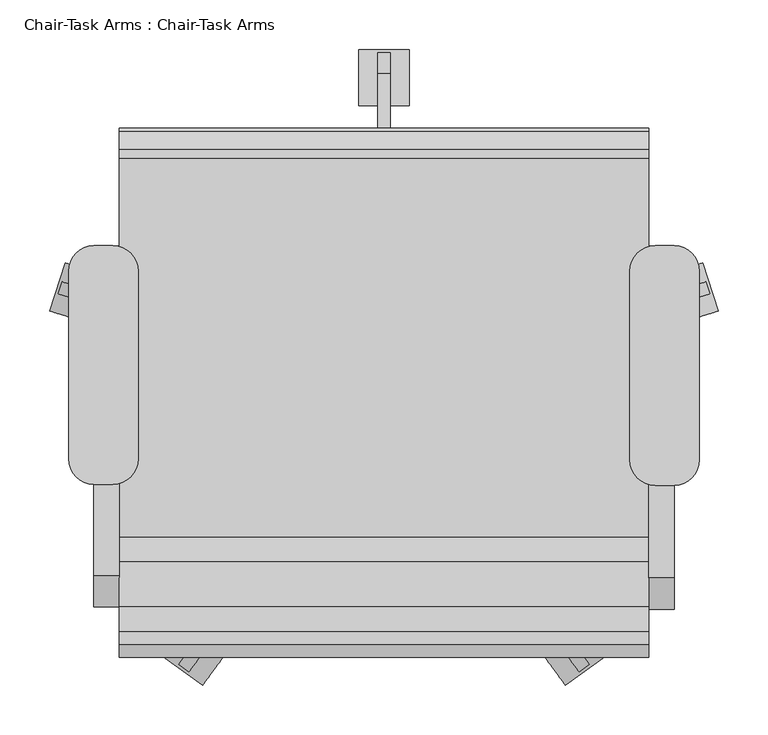
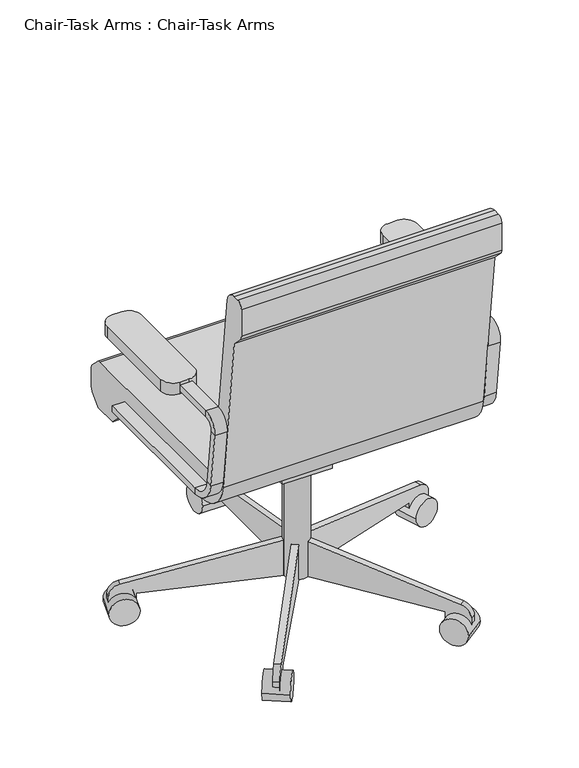
"""IFC4 building model written with IfcOpenShell, lengths in millimetres: furniture geometry, Chair-Task Arms : Chair-Task Arms."""

from ifc_helpers import new_model, si_unit, point, frame, frame_2d, origin, place, context, project, spatial, polyline, circle_curve, trimmed, segment, composite_curve, outline, extrude, source, transform, mapped, element, save
from ifc_brep_helpers import plane_surface, cylinder_surface, revolved_surface, advanced_brep


def chair_task_arms_chair_task_arms_fa5a08ef(model_context):
    return source(origin(), model_context, "Body", "SolidModel", [
        extrude(outline(composite_curve([segment(polyline([(433.0908197, -74.2028048), (414.0408197, -74.2028048)]), True, "CONTINUOUS"), segment(trimmed(circle_curve(frame_2d((414.0408197, -48.8028048)), 25.4), [point((414.0408197, -74.2028048))], [point((388.6408197, -48.8028048))], False, "CARTESIAN"), True, "CONTINUOUS"), segment(polyline([(388.6408197, -48.8028048), (388.6408197, 141.6319091)]), True, "CONTINUOUS"), segment(trimmed(circle_curve(frame_2d((414.0408197, 141.6319091)), 25.4), [point((388.6408197, 141.6319091))], [point((414.0408197, 167.0319091))], False, "CARTESIAN"), True, "CONTINUOUS"), segment(polyline([(414.0408197, 167.0319091), (433.0908197, 167.0319091)]), True, "CONTINUOUS"), segment(trimmed(circle_curve(frame_2d((433.0908197, 141.6319091)), 25.4), [point((433.0908197, 167.0319091))], [point((458.4908197, 141.6319091))], False, "CARTESIAN"), True, "CONTINUOUS"), segment(polyline([(458.4908197, 141.6319091), (458.4908197, -48.8028048)]), True, "CONTINUOUS"), segment(trimmed(circle_curve(frame_2d((433.0908197, -48.8028048)), 25.4), [point((458.4908197, -48.8028048))], [point((433.0908197, -74.2028048))], False, "CARTESIAN"), True, "CONTINUOUS")], self_intersect=False)), frame((0.0, 0.0, 596.9), z_axis=(0.0, 0.0, 1.0), x_axis=(1.0, 0.0, 0.0)), (0.0, 0.0, 1.0), 25.4),
        extrude(outline(composite_curve([segment(polyline([(-132.0591803, -73.1575984), (-151.1091803, -73.1575984)]), True, "CONTINUOUS"), segment(trimmed(circle_curve(frame_2d((-151.1091803, -47.7575984)), 25.4), [point((-151.1091803, -73.1575984))], [point((-176.5091803, -47.7575984))], False, "CARTESIAN"), True, "CONTINUOUS"), segment(polyline([(-176.5091803, -47.7575984), (-176.5091803, 141.6319091)]), True, "CONTINUOUS"), segment(trimmed(circle_curve(frame_2d((-151.1091803, 141.6319091)), 25.4), [point((-176.5091803, 141.6319091))], [point((-151.1091803, 167.0319091))], False, "CARTESIAN"), True, "CONTINUOUS"), segment(polyline([(-151.1091803, 167.0319091), (-132.0591803, 167.0319091)]), True, "CONTINUOUS"), segment(trimmed(circle_curve(frame_2d((-132.0591803, 141.6319091)), 25.4), [point((-132.0591803, 167.0319091))], [point((-106.6591803, 141.6319091))], False, "CARTESIAN"), True, "CONTINUOUS"), segment(polyline([(-106.6591803, 141.6319091), (-106.6591803, -47.7575984)]), True, "CONTINUOUS"), segment(trimmed(circle_curve(frame_2d((-132.0591803, -47.7575984)), 25.4), [point((-106.6591803, -47.7575984))], [point((-132.0591803, -73.1575984))], False, "CARTESIAN"), True, "CONTINUOUS")], self_intersect=False)), frame((0.0, 0.0, 596.9), z_axis=(0.0, 0.0, 1.0), x_axis=(1.0, 0.0, 0.0)), (0.0, 0.0, 1.0), 25.4),
        advanced_brep(
        [(-151.1091803, 167.0319091, 412.75), (-151.1091803, 167.0319091, 425.45), (-125.7091803, 167.0319091, 425.45), (-125.7091803, 167.0319091, 412.75), (-151.1091803, -126.2388651, 412.75), (-151.1091803, -126.2388651, 425.45), (-125.7091803, -126.2388651, 425.45), (-125.7091803, -126.2388651, 412.75), (-151.1091803, -170.3844094, 464.7064065), (-151.1091803, -182.9974221, 463.2225227), (-125.7091803, -170.3844094, 464.7064065), (-125.7091803, -182.9974221, 463.2225227), (-151.1091803, -196.7936301, 580.4902904), (-151.1091803, -184.1806174, 581.9741742), (-125.7091803, -184.1806174, 581.9741742), (-125.7091803, -196.7936301, 580.4902904), (-151.1091803, -165.2610984, 603.25), (-151.1091803, -165.2610984, 615.95), (-125.7091803, -165.2610984, 603.25), (-125.7091803, -165.2610984, 615.95), (-151.1091803, 18.9459016, 615.95), (-125.7091803, 18.9459016, 615.95), (-125.7091803, 18.9459016, 603.25), (-151.1091803, 18.9459016, 603.25)],
        [
            (0, 1),
            (1, 2),
            (2, 3),
            (3, 0),
            (0, 4),
            (4, 5),
            (5, 1),
            (5, 6),
            (6, 2),
            (6, 7),
            (7, 3),
            (7, 4),
            (8, 5, circle_curve(frame((-151.1091803, -126.2388651, 469.9), z_axis=(1.0, 0.0, 0.0), x_axis=(0.0, 0.0, -1.0)), 44.45)),
            (4, 9, circle_curve(frame((-151.1091803, -126.2388651, 469.9), z_axis=(-1.0, 0.0, 0.0), x_axis=(0.0, 0.0, -1.0)), 57.15)),
            (9, 8),
            (10, 6, circle_curve(frame((-125.7091803, -126.2388651, 469.9), z_axis=(1.0, 0.0, 0.0), x_axis=(0.0, 0.0, -1.0)), 44.45)),
            (8, 10),
            (11, 7, circle_curve(frame((-125.7091803, -126.2388651, 469.9), z_axis=(1.0, 0.0, 0.0), x_axis=(0.0, 0.0, -1.0)), 57.15)),
            (10, 11),
            (11, 9),
            (9, 12),
            (12, 13),
            (13, 8),
            (13, 14),
            (14, 10),
            (14, 15),
            (15, 11),
            (15, 12),
            (16, 13, circle_curve(frame((-151.1091803, -165.2610984, 584.2), z_axis=(1.0, 0.0, 0.0), x_axis=(0.0, -0.9931506043228768, -0.11684124756739202)), 19.05)),
            (12, 17, circle_curve(frame((-151.1091803, -165.2610984, 584.2), z_axis=(-1.0, 0.0, 0.0), x_axis=(0.0, -0.9931506043228768, -0.11684124756739202)), 31.75)),
            (17, 16),
            (18, 14, circle_curve(frame((-125.7091803, -165.2610984, 584.2), z_axis=(1.0, 0.0, 0.0), x_axis=(0.0, -0.9931506043228768, -0.11684124756739202)), 19.05)),
            (16, 18),
            (19, 15, circle_curve(frame((-125.7091803, -165.2610984, 584.2), z_axis=(1.0, 0.0, 0.0), x_axis=(0.0, -0.9931506043228768, -0.11684124756739202)), 31.75)),
            (18, 19),
            (19, 17),
            (20, 21),
            (21, 22),
            (22, 23),
            (23, 20),
            (17, 20),
            (23, 16),
            (22, 18),
            (21, 19),
        ],
        [
            plane_surface(frame((-152.608212, 167.0319091, 419.1), z_axis=(0.0, 1.0, 0.0), x_axis=(0.0, 0.0, -1.0))),
            plane_surface(frame((-151.1091803, 167.0319091, 412.75), z_axis=(-1.0, 0.0, 0.0), x_axis=(0.0, -1.0, 0.0))),
            plane_surface(frame((-151.1091803, 167.0319091, 425.45), z_axis=(0.0, 0.0, 1.0), x_axis=(0.0, -1.0, 0.0))),
            plane_surface(frame((-125.7091803, 167.0319091, 425.45), z_axis=(1.0, 0.0, 0.0), x_axis=(0.0, -1.0, 0.0))),
            plane_surface(frame((-125.7091803, 167.0319091, 412.75), z_axis=(0.0, 0.0, -1.0), x_axis=(0.0, -1.0, 0.0))),
            plane_surface(frame((-151.1091803, -126.2388651, 469.9), z_axis=(-1.0, 0.0, 0.0), x_axis=(0.0, 0.0, -1.0))),
            revolved_surface(polyline([(-151.1091803, -126.2388651, 425.45), (-125.7091803, -126.2388651, 425.45)]), (-138.4091803, -126.2388651, 469.9), (-1.0, 0.0, 0.0)),
            plane_surface(frame((-125.7091803, -126.2388651, 469.9), z_axis=(1.0, 0.0, 0.0), x_axis=(0.0, 0.0, -1.0))),
            cylinder_surface(frame((-138.4091803, -126.2388651, 469.9), z_axis=(-1.0, 0.0, 0.0), x_axis=(0.0, 0.0, -1.0)), 57.15),
            plane_surface(frame((-151.1091803, -182.9974221, 463.2225227), z_axis=(-1.0, 0.0, 0.0), x_axis=(0.0, -0.1168412475673856, 0.9931506043228776))),
            plane_surface(frame((-151.1091803, -170.3844094, 464.7064065), z_axis=(0.0, 0.9931506043228776, 0.1168412475673856), x_axis=(0.0, -0.1168412475673856, 0.9931506043228776))),
            plane_surface(frame((-125.7091803, -170.3844094, 464.7064065), z_axis=(1.0, 0.0, 0.0), x_axis=(0.0, -0.1168412475673856, 0.9931506043228776))),
            plane_surface(frame((-125.7091803, -182.9974221, 463.2225227), z_axis=(0.0, -0.9931506043228776, -0.1168412475673856), x_axis=(0.0, -0.1168412475673856, 0.9931506043228776))),
            plane_surface(frame((-151.1091803, -165.2610984, 584.2), z_axis=(-1.0, 0.0, 0.0), x_axis=(0.0, -0.9931506043228768, -0.11684124756739202))),
            revolved_surface(polyline([(-151.1091803, -184.1806174123508, 581.9741742338413), (-125.7091803, -184.1806174123508, 581.9741742338413)]), (-138.4091803, -165.2610984, 584.2), (-1.0, 0.0, 0.0)),
            plane_surface(frame((-125.7091803, -165.2610984, 584.2), z_axis=(1.0, 0.0, 0.0), x_axis=(0.0, -0.9931506043228768, -0.11684124756739202))),
            cylinder_surface(frame((-138.4091803, -165.2610984, 584.2), z_axis=(-1.0, 0.0, 0.0), x_axis=(0.0, -0.9931506043228768, -0.11684124756739202)), 31.75),
            plane_surface(frame((-152.608212, 18.9459016, 609.6), z_axis=(0.0, 1.0, 0.0), x_axis=(0.0, 0.0, 1.0))),
            plane_surface(frame((-151.1091803, -165.2610984, 615.95), z_axis=(-1.0, 0.0, 0.0), x_axis=(0.0, 1.0, 0.0))),
            plane_surface(frame((-151.1091803, -165.2610984, 603.25), z_axis=(0.0, 0.0, -1.0), x_axis=(0.0, 1.0, 0.0))),
            plane_surface(frame((-125.7091803, -165.2610984, 603.25), z_axis=(1.0, 0.0, 0.0), x_axis=(0.0, 1.0, 0.0))),
            plane_surface(frame((-125.7091803, -165.2610984, 615.95), z_axis=(0.0, 0.0, 1.0), x_axis=(0.0, 1.0, 0.0))),
        ],
        [
            (0, [[1, 2, 3, 4]]),
            (1, [[-1, 5, 6, 7]]),
            (2, [[-2, -7, 8, 9]]),
            (3, [[-3, -9, 10, 11]]),
            (4, [[-4, -11, 12, -5]]),
            (5, [[13, -6, 14, 15]]),
            (6, [[16, -8, -13, 17]]),
            (7, [[18, -10, -16, 19]]),
            (8, [[-14, -12, -18, 20]]),
            (9, [[-15, 21, 22, 23]]),
            (10, [[-17, -23, 24, 25]]),
            (11, [[-19, -25, 26, 27]]),
            (12, [[-20, -27, 28, -21]]),
            (13, [[29, -22, 30, 31]]),
            (14, [[32, -24, -29, 33]]),
            (15, [[34, -26, -32, 35]]),
            (16, [[-30, -28, -34, 36]]),
            (17, [[37, 38, 39, 40]]),
            (18, [[-31, 41, -40, 42]]),
            (19, [[-33, -42, -39, 43]]),
            (20, [[-35, -43, -38, 44]]),
            (21, [[-36, -44, -37, -41]]),
        ],
    ),
        advanced_brep(
        [(433.0908197, 167.0319091, 425.45), (433.0908197, 167.0319091, 412.75), (407.6908197, 167.0319091, 412.75), (407.6908197, 167.0319091, 425.45), (433.0908197, -128.329278, 425.45), (433.0908197, -128.329278, 412.75), (407.6908197, -128.329278, 412.75), (407.6908197, -128.329278, 425.45), (433.0908197, -185.0878351, 463.2225227), (433.0908197, -172.4748224, 464.7064065), (407.6908197, -185.0878351, 463.2225227), (407.6908197, -172.4748224, 464.7064065), (433.0908197, -186.2710303, 581.9741742), (433.0908197, -198.884043, 580.4902904), (407.6908197, -198.884043, 580.4902904), (407.6908197, -186.2710303, 581.9741742), (433.0908197, -167.3515113, 615.95), (433.0908197, -167.3515113, 603.25), (407.6908197, -167.3515113, 615.95), (407.6908197, -167.3515113, 603.25), (433.0908197, 18.9459016, 603.25), (407.6908197, 18.9459016, 603.25), (407.6908197, 18.9459016, 615.95), (433.0908197, 18.9459016, 615.95)],
        [
            (0, 1),
            (1, 2),
            (2, 3),
            (3, 0),
            (0, 4),
            (4, 5),
            (5, 1),
            (5, 6),
            (6, 2),
            (6, 7),
            (7, 3),
            (7, 4),
            (8, 5, circle_curve(frame((433.0908197, -128.329278, 469.9), z_axis=(1.0, 0.0, 0.0), x_axis=(0.0, 0.0, -1.0)), 57.15)),
            (4, 9, circle_curve(frame((433.0908197, -128.329278, 469.9), z_axis=(-1.0, 0.0, 0.0), x_axis=(0.0, 0.0, -1.0)), 44.45)),
            (9, 8),
            (10, 6, circle_curve(frame((407.6908197, -128.329278, 469.9), z_axis=(1.0, 0.0, 0.0), x_axis=(0.0, 0.0, -1.0)), 57.15)),
            (8, 10),
            (11, 7, circle_curve(frame((407.6908197, -128.329278, 469.9), z_axis=(1.0, 0.0, 0.0), x_axis=(0.0, 0.0, -1.0)), 44.45)),
            (10, 11),
            (11, 9),
            (9, 12),
            (12, 13),
            (13, 8),
            (13, 14),
            (14, 10),
            (14, 15),
            (15, 11),
            (15, 12),
            (16, 13, circle_curve(frame((433.0908197, -167.3515113, 584.2), z_axis=(1.0, 0.0, 0.0), x_axis=(0.0, -0.9931506043228767, -0.1168412475673929)), 31.75)),
            (12, 17, circle_curve(frame((433.0908197, -167.3515113, 584.2), z_axis=(-1.0, 0.0, 0.0), x_axis=(0.0, -0.9931506043228767, -0.1168412475673929)), 19.05)),
            (17, 16),
            (18, 14, circle_curve(frame((407.6908197, -167.3515113, 584.2), z_axis=(1.0, 0.0, 0.0), x_axis=(0.0, -0.9931506043228767, -0.1168412475673929)), 31.75)),
            (16, 18),
            (19, 15, circle_curve(frame((407.6908197, -167.3515113, 584.2), z_axis=(1.0, 0.0, 0.0), x_axis=(0.0, -0.9931506043228767, -0.1168412475673929)), 19.05)),
            (18, 19),
            (19, 17),
            (20, 21),
            (21, 22),
            (22, 23),
            (23, 20),
            (17, 20),
            (23, 16),
            (22, 18),
            (21, 19),
        ],
        [
            plane_surface(frame((406.191788, 167.0319091, 419.1), z_axis=(0.0, 1.0, 0.0), x_axis=(0.0, 0.0, -1.0))),
            plane_surface(frame((433.0908197, 167.0319091, 425.45), z_axis=(1.0, 0.0, 0.0), x_axis=(0.0, -1.0, 0.0))),
            plane_surface(frame((433.0908197, 167.0319091, 412.75), z_axis=(0.0, 0.0, -1.0), x_axis=(0.0, -1.0, 0.0))),
            plane_surface(frame((407.6908197, 167.0319091, 412.75), z_axis=(-1.0, 0.0, 0.0), x_axis=(0.0, -1.0, 0.0))),
            plane_surface(frame((407.6908197, 167.0319091, 425.45), z_axis=(0.0, 0.0, 1.0), x_axis=(0.0, -1.0, 0.0))),
            plane_surface(frame((433.0908197, -128.329278, 469.9), z_axis=(1.0, 0.0, 0.0), x_axis=(0.0, 0.0, -1.0))),
            cylinder_surface(frame((420.3908197, -128.329278, 469.9), z_axis=(-1.0, 0.0, 0.0), x_axis=(0.0, 0.0, -1.0)), 57.15),
            plane_surface(frame((407.6908197, -128.329278, 469.9), z_axis=(-1.0, 0.0, 0.0), x_axis=(0.0, 0.0, -1.0))),
            revolved_surface(polyline([(407.6908197, -128.329278, 425.45), (433.0908197, -128.329278, 425.45)]), (420.3908197, -128.329278, 469.9), (-1.0, 0.0, 0.0)),
            plane_surface(frame((433.0908197, -172.4748224, 464.7064065), z_axis=(1.0, 0.0, 0.0), x_axis=(0.0, -0.11684124756738626, 0.9931506043228775))),
            plane_surface(frame((433.0908197, -185.0878351, 463.2225227), z_axis=(0.0, -0.9931506043228775, -0.11684124756738655), x_axis=(0.0, -0.11684124756738655, 0.9931506043228775))),
            plane_surface(frame((407.6908197, -185.0878351, 463.2225227), z_axis=(-1.0, 0.0, 0.0), x_axis=(0.0, -0.11684124756738626, 0.9931506043228775))),
            plane_surface(frame((407.6908197, -172.4748224, 464.7064065), z_axis=(0.0, 0.9931506043228775, 0.11684124756738626), x_axis=(0.0, -0.11684124756738626, 0.9931506043228775))),
            plane_surface(frame((433.0908197, -167.3515113, 584.2), z_axis=(1.0, 0.0, 0.0), x_axis=(0.0, -0.9931506043228767, -0.1168412475673929))),
            cylinder_surface(frame((420.3908197, -167.3515113, 584.2), z_axis=(-1.0, 0.0, 0.0), x_axis=(0.0, -0.9931506043228767, -0.1168412475673929)), 31.75),
            plane_surface(frame((407.6908197, -167.3515113, 584.2), z_axis=(-1.0, 0.0, 0.0), x_axis=(0.0, -0.9931506043228767, -0.1168412475673929))),
            revolved_surface(polyline([(407.6908197, -186.2710303123508, 581.9741742338412), (433.0908197, -186.2710303123508, 581.9741742338412)]), (420.3908197, -167.3515113, 584.2), (-1.0, 0.0, 0.0)),
            plane_surface(frame((406.191788, 18.9459016, 609.6), z_axis=(0.0, 1.0, 0.0), x_axis=(0.0, 0.0, 1.0))),
            plane_surface(frame((433.0908197, -167.3515113, 603.25), z_axis=(1.0, 0.0, 0.0), x_axis=(0.0, 1.0, 0.0))),
            plane_surface(frame((433.0908197, -167.3515113, 615.95), z_axis=(0.0, 0.0, 1.0), x_axis=(0.0, 1.0, 0.0))),
            plane_surface(frame((407.6908197, -167.3515113, 615.95), z_axis=(-1.0, 0.0, 0.0), x_axis=(0.0, 1.0, 0.0))),
            plane_surface(frame((407.6908197, -167.3515113, 603.25), z_axis=(0.0, 0.0, -1.0), x_axis=(0.0, 1.0, 0.0))),
        ],
        [
            (0, [[1, 2, 3, 4]]),
            (1, [[-1, 5, 6, 7]]),
            (2, [[-2, -7, 8, 9]]),
            (3, [[-3, -9, 10, 11]]),
            (4, [[-4, -11, 12, -5]]),
            (5, [[13, -6, 14, 15]]),
            (6, [[16, -8, -13, 17]]),
            (7, [[18, -10, -16, 19]]),
            (8, [[-14, -12, -18, 20]]),
            (9, [[-15, 21, 22, 23]]),
            (10, [[-17, -23, 24, 25]]),
            (11, [[-19, -25, 26, 27]]),
            (12, [[-20, -27, 28, -21]]),
            (13, [[29, -22, 30, 31]]),
            (14, [[32, -24, -29, 33]]),
            (15, [[34, -26, -32, 35]]),
            (16, [[-30, -28, -34, 36]]),
            (17, [[37, 38, 39, 40]]),
            (18, [[-31, 41, -40, 42]]),
            (19, [[-33, -42, -39, 43]]),
            (20, [[-35, -43, -38, 44]]),
            (21, [[-36, -44, -37, -41]]),
        ],
    ),
        extrude(outline(composite_curve([segment(trimmed(circle_curve(frame_2d((140.9908197, 18.9459016)), 25.4), [point((115.5908197, 18.9459016))], [point((166.3908197, 18.9459016))], False, "CARTESIAN"), True, "CONTINUOUS"), segment(trimmed(circle_curve(frame_2d((140.9908197, 18.9459016)), 25.4), [point((166.3908197, 18.9459016))], [point((115.5908197, 18.9459016))], False, "CARTESIAN"), True, "CONTINUOUS")], self_intersect=False)), frame((0.0, 0.0, 53.5835944), z_axis=(0.0, 0.0, 1.0), x_axis=(1.0, 0.0, 0.0)), (0.0, 0.0, 1.0), 330.5914056),
        extrude(outline(composite_curve([segment(trimmed(circle_curve(frame_2d((0.0, -28.2002727)), 28.2002727), [point((0.0, -56.4005455))], [point((0.0, 0.0))], False, "CARTESIAN"), True, "CONTINUOUS"), segment(trimmed(circle_curve(frame_2d((0.0, -28.2002727)), 28.2002727), [point((0.0, 0.0))], [point((0.0, -56.4005455))], False, "CARTESIAN"), True, "CONTINUOUS")], self_intersect=False)), frame((477.6203484, 101.6163254, 28.1835944), z_axis=(-0.3090169943749423, 0.9510565162951553, 0.0), x_axis=(0.0, 0.0, 1.0)), (0.0, 0.0, 1.0), 50.8),
        extrude(outline(composite_curve([segment(polyline([(-25.4, 0.0), (0.0, 0.0), (0.0, -50.8), (-24.303053, -50.8)]), True, "CONTINUOUS"), segment(trimmed(circle_curve(frame_2d((-24.303053, -25.4)), 25.4), [point((-24.303053, -50.8))], [point((-49.3171699, -29.8106637))], False, "CARTESIAN"), True, "CONTINUOUS"), segment(polyline([(-49.3171699, -29.8106637), (-101.6, 266.7), (-101.6, 292.1), (-25.4, 292.1), (-25.4, 0.0)]), True, "CONTINUOUS")], self_intersect=False)), frame((420.756686, 103.1705568, 28.1835944), z_axis=(-0.3090169943749423, 0.9510565162951553, 0.0), x_axis=(0.0, 0.0, -1.0)), (0.0, 0.0, 1.0), 12.7),
        extrude(outline(composite_curve([segment(trimmed(circle_curve(frame_2d((0.0, -28.2002727)), 28.2002727), [point((0.0, -56.4005455))], [point((0.0, 0.0))], False, "CARTESIAN"), True, "CONTINUOUS"), segment(trimmed(circle_curve(frame_2d((0.0, -28.2002727)), 28.2002727), [point((0.0, 0.0))], [point((0.0, -56.4005455))], False, "CARTESIAN"), True, "CONTINUOUS")], self_intersect=False)), frame((323.63931, -275.6612394, 28.1835944), z_axis=(0.8090169943749499, 0.5877852522924699, 0.0), x_axis=(0.0, 0.0, 1.0)), (0.0, 0.0, 1.0), 50.8),
        extrude(outline(composite_curve([segment(polyline([(-25.4, 0.0), (0.0, 0.0), (0.0, -50.8), (-24.303053, -50.8)]), True, "CONTINUOUS"), segment(trimmed(circle_curve(frame_2d((-24.303053, -25.3999999)), 25.4), [point((-24.303053, -50.8))], [point((-49.3171699, -29.8106636))], False, "CARTESIAN"), True, "CONTINUOUS"), segment(polyline([(-49.3171699, -29.8106636), (-101.6, 266.7), (-101.6, 292.1), (-25.4, 292.1), (-25.4, 0.0)]), True, "CONTINUOUS")], self_intersect=False)), frame((307.545634, -221.1003988, 28.1835944), z_axis=(0.8090169943749499, 0.5877852522924699, 0.0), x_axis=(0.0, 0.0, -1.0)), (0.0, 0.0, 1.0), 12.7),
        extrude(outline(composite_curve([segment(trimmed(circle_curve(frame_2d((0.0, -28.2002727)), 28.2002727), [point((0.0, -56.4005455))], [point((0.0, 0.0))], False, "CARTESIAN"), True, "CONTINUOUS"), segment(trimmed(circle_curve(frame_2d((0.0, -28.2002727)), 28.2002727), [point((0.0, 0.0))], [point((0.0, -56.4005455))], False, "CARTESIAN"), True, "CONTINUOUS")], self_intersect=False)), frame((-41.6576707, -275.6612394, 28.1835944), z_axis=(-0.8090169943749458, 0.5877852522924754, 0.0), x_axis=(0.0, 0.0, -1.0)), (0.0, 0.0, 1.0), 50.8),
        extrude(outline(composite_curve([segment(polyline([(25.4, 0.0), (25.4, 292.1), (101.6, 292.1), (101.6, 266.7), (49.3171699, -29.8106637)]), True, "CONTINUOUS"), segment(trimmed(circle_curve(frame_2d((24.303053, -25.3999999)), 25.4), [point((49.3171699, -29.8106637))], [point((24.303053, -50.8))], False, "CARTESIAN"), True, "CONTINUOUS"), segment(polyline([(24.303053, -50.8), (0.0, -50.8), (0.0, 0.0), (25.4, 0.0)]), True, "CONTINUOUS")], self_intersect=False)), frame((-25.5639946, -221.1003988, 28.1835944), z_axis=(-0.8090169943749459, 0.5877852522924754, 0.0), x_axis=(0.0, 0.0, 1.0)), (0.0, 0.0, 1.0), 12.7),
        extrude(outline(composite_curve([segment(trimmed(circle_curve(frame_2d((0.0, -28.2002727)), 28.2002727), [point((0.0, -56.4005454))], [point((0.0, 0.0))], False, "CARTESIAN"), True, "CONTINUOUS"), segment(trimmed(circle_curve(frame_2d((0.0, -28.2002727)), 28.2002727), [point((0.0, 0.0))], [point((0.0, -56.4005454))], False, "CARTESIAN"), True, "CONTINUOUS")], self_intersect=False)), frame((-195.638709, 101.6163254, 28.1835944), z_axis=(0.3090169943749487, 0.9510565162951532, 0.0), x_axis=(0.0, 0.0, -1.0)), (0.0, 0.0, 1.0), 50.8),
        extrude(outline(composite_curve([segment(polyline([(25.4, 0.0), (25.4, 292.1000001), (101.6, 292.1000001), (101.6, 266.7), (49.3171699, -29.8106636)]), True, "CONTINUOUS"), segment(trimmed(circle_curve(frame_2d((24.303053, -25.4)), 25.4), [point((49.3171699, -29.8106636))], [point((24.303053, -50.8))], False, "CARTESIAN"), True, "CONTINUOUS"), segment(polyline([(24.303053, -50.8), (0.0, -50.8), (0.0, 0.0), (25.4, 0.0)]), True, "CONTINUOUS")], self_intersect=False)), frame((-138.7750467, 103.1705568, 28.1835944), z_axis=(0.3090169943749487, 0.9510565162951532, 0.0), x_axis=(0.0, 0.0, 1.0)), (0.0, 0.0, 1.0), 12.7),
        extrude(outline(composite_curve([segment(trimmed(circle_curve(frame_2d((336.4459016, 28.1835944)), 28.2002727), [point((308.2456289, 28.1835944))], [point((364.6461744, 28.1835944))], False, "CARTESIAN"), True, "CONTINUOUS"), segment(trimmed(circle_curve(frame_2d((336.4459016, 28.1835944)), 28.2002727), [point((364.6461744, 28.1835944))], [point((308.2456289, 28.1835944))], False, "CARTESIAN"), True, "CONTINUOUS")], self_intersect=False)), frame((115.5908197, 0.0, 0.0), z_axis=(1.0, 0.0, 0.0), x_axis=(0.0, 1.0, 0.0)), (0.0, 0.0, 1.0), 50.8),
        extrude(outline(composite_curve([segment(polyline([(311.0459016, 53.5835944), (18.9459016, 53.5835944), (18.9459016, 129.7835944), (44.3459016, 129.7835944), (340.8565654, 77.5007643)]), True, "CONTINUOUS"), segment(trimmed(circle_curve(frame_2d((336.4459016, 52.4866474)), 25.4), [point((340.8565654, 77.5007643))], [point((361.8459016, 52.4866474))], False, "CARTESIAN"), True, "CONTINUOUS"), segment(polyline([(361.8459016, 52.4866474), (361.8459016, 28.1835944), (311.0459016, 28.1835944), (311.0459016, 53.5835944)]), True, "CONTINUOUS")], self_intersect=False)), frame((134.6408197, 0.0, 0.0), z_axis=(1.0, 0.0, 0.0), x_axis=(0.0, 1.0, 0.0)), (0.0, 0.0, 1.0), 12.7),
        extrude(outline(polyline([(69.7459016, 383.7835944), (69.7459016, 371.0835944), (18.9459016, 283.0954134), (-19.1540984, 283.0954134), (-19.1540984, 383.7835944), (69.7459016, 383.7835944)])), frame((90.1908197, 0.0, 0.0), z_axis=(1.0, 0.0, 0.0), x_axis=(0.0, 1.0, 0.0)), (0.0, 0.0, 1.0), 101.6),
        extrude(outline(composite_curve([segment(polyline([(-126.2050455, 457.2), (255.0102301, 457.2)]), True, "CONTINUOUS"), segment(trimmed(circle_curve(frame_2d((255.0102301, 444.5)), 12.7), [point((255.0102301, 457.2))], [point((263.9604301, 453.510212))], False, "CARTESIAN"), True, "CONTINUOUS"), segment(polyline([(263.9604301, 453.510212), (281.8961016, 435.6939999)]), True, "CONTINUOUS"), segment(trimmed(circle_curve(frame_2d((272.9459016, 426.6837879)), 12.7), [point((281.8961016, 435.6939999))], [point((285.6459016, 426.6837879))], False, "CARTESIAN"), True, "CONTINUOUS"), segment(polyline([(285.6459016, 426.6837879), (285.6459016, 391.6405184)]), True, "CONTINUOUS"), segment(trimmed(circle_curve(frame_2d((260.2459016, 391.6405184)), 25.4), [point((285.6459016, 391.6405184))], [point((278.2663256, 373.7401184))], False, "CARTESIAN"), True, "CONTINUOUS"), segment(polyline([(278.2663256, 373.7401184), (260.2470284, 355.6), (209.4470284, 355.6), (181.0744602, 383.7835944), (-107.1089978, 383.7835944)]), True, "CONTINUOUS"), segment(trimmed(circle_curve(frame_2d((-107.1089978, 459.9835944)), 76.2), [point((-107.1089978, 383.7835944))], [point((-182.7870738, 451.0802913))], False, "CARTESIAN"), True, "CONTINUOUS"), segment(polyline([(-182.7870738, 451.0802913), (-222.3540984, 787.4), (-244.0343545, 809.0802561)]), True, "CONTINUOUS"), segment(trimmed(circle_curve(frame_2d((-235.0540984, 818.0605122)), 12.7), [point((-244.0343545, 809.0802561))], [point((-247.7540984, 818.0605122))], False, "CARTESIAN"), True, "CONTINUOUS"), segment(polyline([(-247.7540984, 818.0605122), (-247.7540984, 876.3)]), True, "CONTINUOUS"), segment(trimmed(circle_curve(frame_2d((-235.0540984, 876.3)), 12.7), [point((-247.7540984, 876.3))], [point((-235.0540984, 889.0))], False, "CARTESIAN"), True, "CONTINUOUS"), segment(polyline([(-235.0540984, 889.0), (-222.1789239, 889.0)]), True, "CONTINUOUS"), segment(trimmed(circle_curve(frame_2d((-222.1789239, 863.6)), 25.4), [point((-222.1789239, 889.0))], [point((-196.9528985, 866.5677677))], False, "CARTESIAN"), True, "CONTINUOUS"), segment(polyline([(-196.9528985, 866.5677677), (-151.4310708, 479.6322323)]), True, "CONTINUOUS"), segment(trimmed(circle_curve(frame_2d((-126.2050455, 482.6)), 25.4), [point((-151.4310708, 479.6322323))], [point((-126.2050455, 457.2))], True, "CARTESIAN"), True, "CONTINUOUS")], self_intersect=False)), frame((-125.7091803, 0.0, 0.0), z_axis=(1.0, 0.0, 0.0), x_axis=(0.0, 1.0, 0.0)), (0.0, 0.0, 1.0), 533.4),
    ])


if __name__ == "__main__":
    model = new_model("IFC4")
    model_context = context("Model", 3, world=origin())
    ifc_project = project(units=[si_unit("LENGTHUNIT", "METRE", prefix="MILLI")], contexts=[model_context])
    site = spatial("IfcSite", under=ifc_project)
    building = spatial("IfcBuilding", under=site)
    placement = place(None, origin())
    chair_task_arms_chair_task_arms_shape = chair_task_arms_chair_task_arms_fa5a08ef(model_context)
    element("IfcFurniture", 1, ObjectType="Chair-Task Arms : Chair-Task Arms", at=placement, inside=building, context=model_context, shape_type="MappedRepresentation", body=[
        mapped(chair_task_arms_chair_task_arms_shape, transform((0.0, 0.0, 0.0), x_axis=(1.0, 0.0, 0.0), y_axis=(0.0, 1.0, 0.0), z_axis=(0.0, 0.0, 1.0))),
    ])
    save(model, "model.ifc")

# Revit data of these elements
# Type "Chair-Task Arms : Chair-Task Arms"
#   Assembly Code = "E2020200"
#   Base Material = Plastic, Opaque Black
#   Caster Material = Plastic, Opaque Black
#   Seat/Back Material = Textile - Slate Blue
#   Default Elevation = 0
# Element 1 (IfcFurniture, "Chair-Task Arms : Chair-Task Arms")
#   Materials on its faces: "Plastic, Opaque Black", "Textile - Slate Blue"
# Materials
#   "Plastic, Opaque Black": class "Plastic", colour RGB 0 0 0, transparency 0, Description = "Plastic, generic, opaque black", Cost = 0
#   "Textile - Slate Blue": class "Fabric", colour RGB 98 102 118, transparency 0
